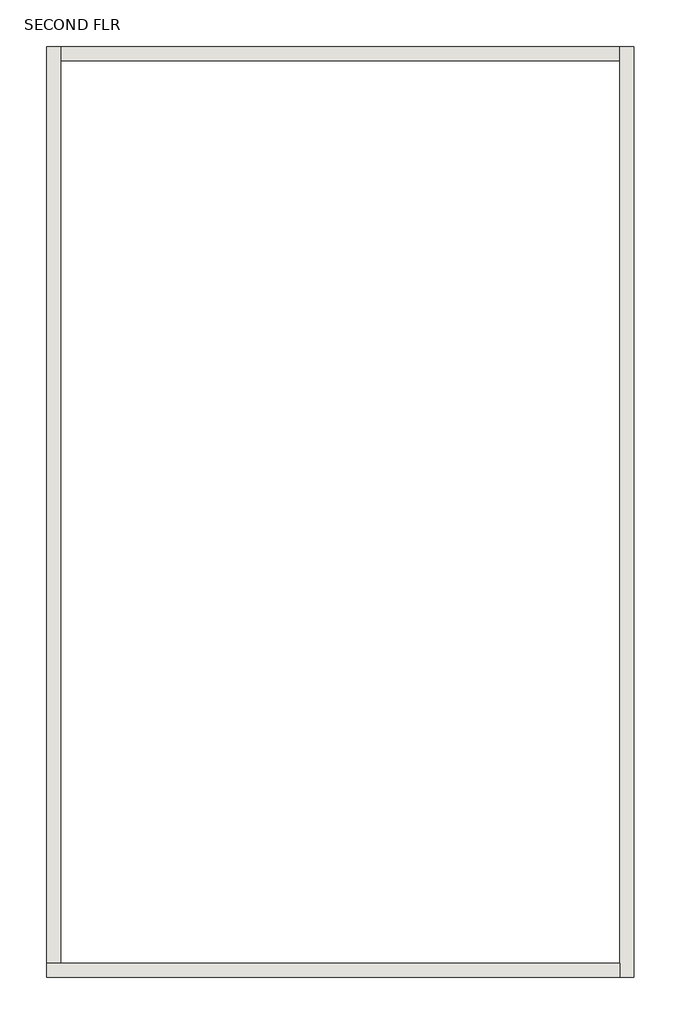
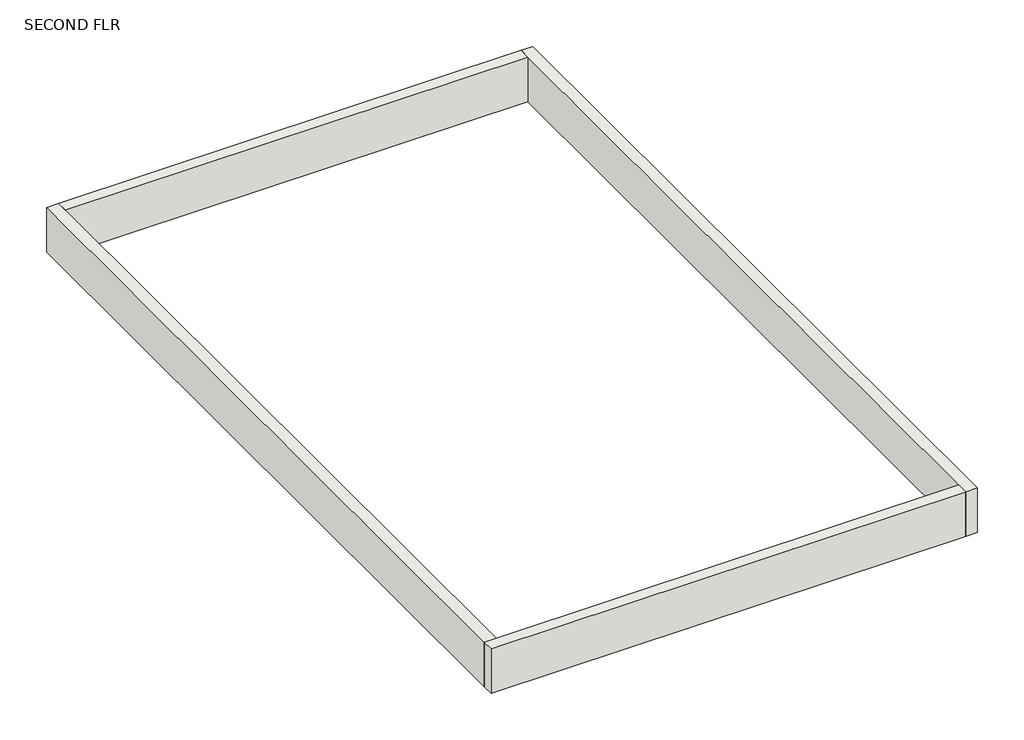
# One storey: 4 walls.
"""IFC4 building model written with IfcOpenShell, lengths in millimetres."""

from ifc_helpers import new_model, si_unit, frame, origin, place, context, project, spatial, polyline, outline, extrude, faceted_brep, element, save

model = new_model("IFC4")

# Units and contexts
model_context = context("Model", 3, world=origin())
ifc_project = project(units=[si_unit("LENGTHUNIT", "METRE", prefix="MILLI")], contexts=[model_context])

# Site, building, storey
site = spatial("IfcSite", under=ifc_project)
building = spatial("IfcBuilding", under=site)
storey = spatial("IfcBuildingStorey", under=building, Name="SECOND FLR", Elevation=6400.8)

# Walls
placement = place(None, origin())
element("IfcWall", 1, ObjectType="EXTERIOR WALL 9\"", at=placement, inside=storey, context=model_context, shape_type="Brep", body=[
    faceted_brep([(-9153.5229553, 7897.0964313, 6400.8), (-9153.5229553, 7668.4964313, 6400.8), (-9153.5229553, -6834.9035687, 6400.8), (-9153.5229553, -7063.5035687, 6400.8), (-9153.5229553, -7063.5035687, 7315.2), (-9153.5229553, -6834.9035687, 7315.2), (-9153.5229553, 7668.4964313, 7315.2), (-9153.5229553, 7897.0964313, 7315.2), (-8924.9229553, 7897.0964313, 6400.8), (-8924.9229553, 7897.0964313, 7315.2), (-8924.9229553, -7063.5035687, 7315.2), (-8924.9229553, -7063.5035687, 6400.8)], [[[0, 1, 2, 3, 4, 5, 6, 7]], [[8, 9, 10, 11]], [[3, 2, 1, 0, 8, 11]], [[7, 6, 5, 4, 10, 9]], [[4, 3, 11, 10]], [[0, 7, 9, 8]]]),
])
element("IfcWall", 2, ObjectType="EXTERIOR WALL 9\"", at=placement, inside=storey, context=model_context, shape_type="Brep", body=[
    faceted_brep([(-9153.5229553, -6834.9035687, 6400.8), (-18145.1229553, -6834.9035687, 6400.8), (-18373.7229553, -6834.9035687, 6400.8), (-18373.7229553, -6834.9035687, 7315.2), (-18145.1229553, -6834.9035687, 7315.2), (-9153.5229553, -6834.9035687, 7315.2), (-9153.5229553, -7063.5035687, 6400.8), (-9153.5229553, -7063.5035687, 7315.2), (-18373.7229553, -7063.5035687, 7315.2), (-18373.7229553, -7063.5035687, 6400.8)], [[[0, 1, 2, 3, 4, 5]], [[6, 7, 8, 9]], [[2, 1, 0, 6, 9]], [[5, 4, 3, 8, 7]], [[0, 5, 7, 6]], [[3, 2, 9, 8]]]),
])
element("IfcWall", 3, ObjectType="EXTERIOR WALL 9\"", at=placement, inside=storey, context=model_context, shape_type="Brep", body=[
    faceted_brep([(-18145.1229553, -6834.9035687, 6400.8), (-18145.1229553, 7668.4964313, 6400.8), (-18145.1229553, 7897.0964313, 6400.8), (-18145.1229553, 7897.0964313, 7315.2), (-18145.1229553, 7668.4964313, 7315.2), (-18145.1229553, -6834.9035687, 7315.2), (-18373.7229553, -6834.9035687, 6400.8), (-18373.7229553, -6834.9035687, 7315.2), (-18373.7229553, 7897.0964313, 7315.2), (-18373.7229553, 7897.0964313, 6400.8)], [[[0, 1, 2, 3, 4, 5]], [[6, 7, 8, 9]], [[2, 1, 0, 6, 9]], [[5, 4, 3, 8, 7]], [[0, 5, 7, 6]], [[3, 2, 9, 8]]]),
])
element("IfcWall", 4, ObjectType="EXTERIOR WALL 9\"", at=placement, inside=storey, context=model_context, shape_type="SweptSolid", body=[
    extrude(outline(polyline([(-9153.5229553, 7668.4964313), (-18145.1229553, 7668.4964313), (-18145.1229553, 7897.0964313), (-9153.5229553, 7897.0964313), (-9153.5229553, 7668.4964313)])), frame((0.0, 0.0, 6400.8), z_axis=(0.0, 0.0, 1.0), x_axis=(1.0, 0.0, 0.0)), (0.0, 0.0, 1.0), 914.4),
])

save(model, "model.ifc")

# Revit data of these elements
# Type "EXTERIOR WALL 9\""
#   Assembly Code = "B2010"
#   Layers, outside or top first: 0' - 9" "EXTERIOR WALL WHITE COLOUR" (function 1)
# Elements 1, 2, 3, 4 (IfcWall, "EXTERIOR WALL 9\"")
#   Top Offset = 0' - 0"
#   Base Offset = 0' - 0"
#   Unconnected Height = 3' - 0"
#   wall height = 3' - 0"
#   Phase Created = New Construction
#   Base Constraint = SECOND FLR
#   Materials on its faces: "EXTERIOR WALL WHITE COLOUR"
# Materials
#   "EXTERIOR WALL WHITE COLOUR": class "Generic", colour RGB 120 120 120, transparency 0, Cost = 0
